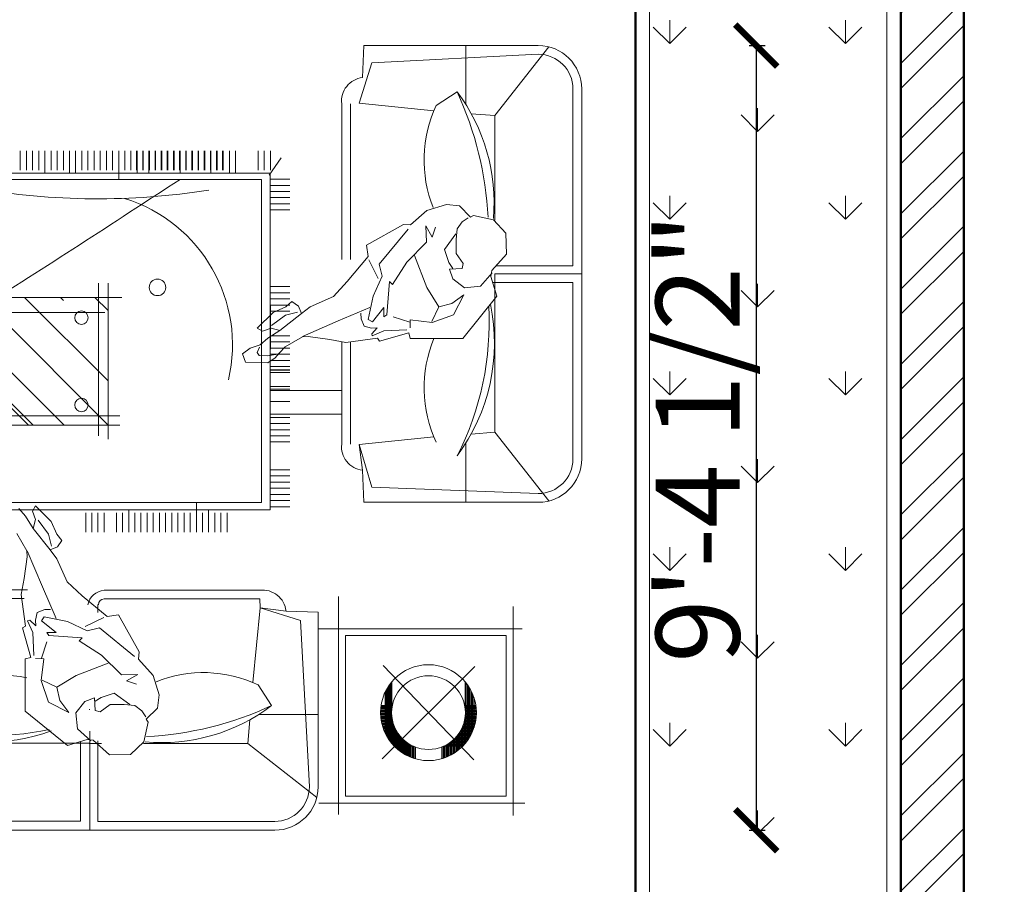
# Model space of a CAD drawing. Units: inches. Extents: x 261 to 2725, y 291 to 1454.
# Tile 31 of 35: x 2359 to 2500, y 546 to 670. Entities that reach past the tile are written whole.
import ezdxf

# ---------------------------------------------------------------- set-up
doc = ezdxf.new("R2010")
doc.units = ezdxf.units.IN
for name, color, linetype, lineweight in [('A-ANNO-DIMS', 136, 'Continuous', 18), ('A-FURN', 30, 'Continuous', 18), ('A-PLNT', 3, 'Continuous', 18), ('A-PLNT-PATT', 3, 'Continuous', 13), ('A-WALL', 222, 'Continuous', 50), ('A-WALL-PATT', 243, 'Continuous', 13)]:
    doc.layers.add(name, color=color, linetype=linetype, lineweight=lineweight)
doc.styles.get("Standard").update_dxf_attribs({"font": 'arial.ttf'})
doc.dimstyles.new('ISO-25', dxfattribs={"dimtxt": 12, "dimasz": 6, "dimexe": 1.25, "dimexo": 0.625, "dimtad": 1, "dimdec": 0, "dimlunit": 3, "dimtxsty": 'Standard', "dimblk": 'ARCHTICK', "dimcen": 2.5, "dimadec": 0, "dimazin": 0, "dimtfac": 1, "dimtdec": 0, "dimtmove": 0, "dimatfit": 3, "dimfxl": 1, "dimfxlon": 1, "dimarcsym": 0})

# ---------------------------------------------------------------- blocks, each defined once
blk = doc.blocks.new('A$C4DC51D13')
for p, q in [((3265.3, 2996.2), (1188.4, 2996.2)), ((2559.6, 2996.2), (2559.6, 2617.8)), ((1928.3, 2961.6), (2524.2, 2961.6)), ((2524.2, 2961.6), (2524.2, 2658.6)), ((2590.4, 2962.7), (2590.4, 2654.5)), ((3265.3, 2962.7), (2590.4, 2962.7)), ((3509.6, 2103.5), (3509.6, 2936.7)), ((4175.2, 2939.6), (4175.2, 2141.8)), ((3163.3, 2664.8), (3425.7, 2870.9)), ((3434.4, 2892.3), (4220.4, 2892.3)), ((3536.2, 2253.3), (3536.2, 2865.7)), ((3536.2, 2865.7), (4148.5, 2865.7)), ((4148.5, 2865.7), (4148.5, 2253.3)), ((3397.7, 2830.3), (3364.5, 2194.8)), ((3430.8, 2163.8), (3430.8, 2830.3)), ((4028.9, 2370.8), (3676, 2723.7)), ((4025.2, 2727.4), (3679.8, 2367.1)), ((3763, 2655.8), (3763, 2706.9)), ((3764.4, 2657), (3764.4, 2707.7)), ((3767.2, 2659.2), (3767.2, 2709.2)), ((3768.7, 2660.3), (3768.7, 2709.9)), ((3771.5, 2662.3), (3771.5, 2711.3)), ((3772.9, 2663.3), (3772.9, 2712)), ((3775.7, 2665.1), (3775.7, 2713.4)), ((3777.1, 2666.1), (3777.1, 2714)), ((3779.9, 2667.8), (3779.9, 2715.2)), ((3781.4, 2668.6), (3781.4, 2715.9)), ((3784.1, 2670.2), (3784.1, 2717)), ((3785.6, 2671), (3785.6, 2717.6)), ((3789.8, 2673.2), (3789.8, 2719.2)), ((3794, 2675.2), (3794, 2720.7)), ((3798.3, 2677.1), (3798.3, 2722)), ((3802.5, 2678.8), (3802.5, 2723.3)), ((3903.9, 2678.2), (3903.9, 2722.9)), ((3908.1, 2676.5), (3908.1, 2721.6)), ((3912.4, 2674.6), (3912.4, 2720.2)), ((3916.6, 2672.5), (3916.6, 2718.7)), ((3920.8, 2670.2), (3920.8, 2717)), ((3925.1, 2667.8), (3925.1, 2715.2)), ((3929.3, 2665.1), (3929.3, 2713.4)), ((3933.5, 2662.3), (3933.5, 2711.3)), ((3937.7, 2659.2), (3937.7, 2709.2)), ((3942, 2655.8), (3942, 2706.9)), ((3716.5, 2583.3), (3716.5, 2669.7)), ((3718, 2588.4), (3718, 2671.3)), ((3718.1, 2671.5), (3786.5, 2671.5)), ((3786.5, 2671.5), (3718.1, 2671.5)), ((3720.7, 2596.6), (3720.7, 2674.3)), ((3722.2, 2600.3), (3722.2, 2675.7)), ((3795.2, 2675.7), (3722.2, 2675.7)), ((3725, 2606.7), (3725, 2678.5)), ((3726.4, 2609.7), (3726.4, 2679.9)), ((3729.2, 2615), (3729.2, 2682.5)), ((3730.6, 2617.6), (3730.6, 2683.8)), ((3733.4, 2622.2), (3733.4, 2686.2)), ((3734.9, 2624.4), (3734.9, 2687.4)), ((3737.6, 2628.5), (3737.6, 2689.7)), ((3739.1, 2630.5), (3739.1, 2690.9)), ((3741.9, 2634.2), (3741.9, 2693)), ((3743.3, 2636), (3743.3, 2694.1)), ((3746.1, 2639.3), (3746.1, 2696.1)), ((3747.5, 2641), (3747.5, 2697.2)), ((3750.3, 2644), (3750.3, 2699.1)), ((3751.8, 2645.5), (3751.8, 2700)), ((3754.5, 2648.3), (3754.5, 2701.8)), ((3756, 2649.6), (3756, 2702.7)), ((3758.8, 2652.2), (3758.8, 2704.4)), ((3760.2, 2653.5), (3760.2, 2705.3)), ((3982.8, 2675.7), (3909.8, 2675.7)), ((3986.8, 2671.5), (3918.5, 2671.5)), ((3946.2, 2652.2), (3946.2, 2704.4)), ((3950.4, 2648.3), (3950.4, 2701.8)), ((3954.6, 2644), (3954.6, 2699.1)), ((3958.9, 2639.3), (3958.9, 2696.1)), ((3963.1, 2634.2), (3963.1, 2693)), ((3967.3, 2628.5), (3967.3, 2689.7)), ((3971.5, 2622.2), (3971.5, 2686.2)), ((3975.8, 2615), (3975.8, 2682.5)), ((3980, 2606.7), (3980, 2678.5)), ((3984.2, 2596.6), (3984.2, 2674.3)), ((3988.5, 2583.3), (3988.5, 2669.7)), ((1895.2, 2663.7), (2557.3, 2663.7)), ((2603.6, 2664.8), (2559, 2664.8)), ((3163.3, 2664.8), (2764.7, 2664.8)), ((3170.4, 2574.2), (3163.3, 2664.8)), ((3691.1, 2460.9), (3691.1, 2633.6)), ((3691.1, 2633.5), (3741.3, 2633.5)), ((3741.3, 2633.5), (3691.1, 2633.5)), ((3692.6, 2458.3), (3692.6, 2636.3)), ((3693.4, 2637.7), (3744.7, 2637.7)), ((3744.7, 2637.7), (3693.4, 2637.7)), ((3695.4, 2453.4), (3695.4, 2641.1)), ((3695.9, 2641.9), (3748.4, 2641.9)), ((3748.4, 2641.9), (3695.9, 2641.9)), ((3696.8, 2451.1), (3696.8, 2643.5)), ((3698.5, 2646.1), (3752.4, 2646.1)), ((3752.4, 2646.1), (3698.5, 2646.1)), ((3699.6, 2446.7), (3699.6, 2647.8)), ((3701, 2444.5), (3701, 2650)), ((3701.3, 2650.4), (3756.8, 2650.4)), ((3756.8, 2650.4), (3701.3, 2650.4)), ((3703.8, 2440.6), (3703.8, 2654)), ((3704.3, 2654.6), (3761.5, 2654.6)), ((3761.5, 2654.6), (3704.3, 2654.6)), ((3705.3, 2438.6), (3705.3, 2656)), ((3707.4, 2658.8), (3766.8, 2658.8)), ((3766.8, 2658.8), (3707.4, 2658.8)), ((3708.1, 2434.9), (3708.1, 2659.6)), ((3709.5, 2433.1), (3709.5, 2661.5)), ((3710.8, 2663.1), (3772.6, 2663.1)), ((3772.6, 2663.1), (3710.8, 2663.1)), ((3712.3, 2558.8), (3712.3, 2664.9)), ((3713.7, 2570.4), (3713.7, 2666.6)), ((3714.3, 2667.3), (3779.1, 2667.3)), ((3779.1, 2667.3), (3714.3, 2667.3)), ((3990.6, 2667.3), (3925.9, 2667.3)), ((3994.2, 2663.1), (3932.4, 2663.1)), ((3997.5, 2658.8), (3938.2, 2658.8)), ((4000.7, 2654.6), (3943.4, 2654.6)), ((4003.7, 2650.4), (3948.2, 2650.4)), ((4006.5, 2646.1), (3952.5, 2646.1)), ((4009.1, 2641.9), (3956.5, 2641.9)), ((4011.6, 2637.7), (3960.2, 2637.7)), ((3963.1, 2667.3), (3963.1, 2633.5)), ((4013.9, 2633.5), (3963.7, 2633.5)), ((3992.7, 2558.8), (3992.7, 2664.9)), ((3996.9, 2434.9), (3996.9, 2659.6)), ((4001.1, 2440.6), (4001.1, 2654)), ((4005.4, 2446.7), (4005.4, 2647.8)), ((4009.6, 2453.4), (4009.6, 2641.1)), ((4013.8, 2460.9), (4013.8, 2633.6)), ((3675.9, 2595.4), (3720.3, 2595.4)), ((3677.2, 2599.7), (3721.9, 2599.7)), ((3678.5, 2603.9), (3723.7, 2603.9)), ((3679.9, 2608.1), (3725.6, 2608.1)), ((3681.5, 2612.3), (3727.8, 2612.3)), ((3683.1, 2616.6), (3730.1, 2616.6)), ((3684.9, 2620.8), (3732.5, 2620.8)), ((3686.8, 2625), (3735.2, 2625)), ((3686.9, 2469.3), (3686.9, 2625.2)), ((3688.4, 2466.3), (3688.4, 2628.2)), ((3688.9, 2629.2), (3738.2, 2629.2)), ((3738.2, 2629.2), (3688.9, 2629.2)), ((4016.1, 2629.2), (3966.8, 2629.2)), ((4018.1, 2625), (3969.7, 2625)), ((4020, 2620.8), (3972.4, 2620.8)), ((4021.8, 2616.6), (3974.9, 2616.6)), ((4023.5, 2612.3), (3977.2, 2612.3)), ((4025.1, 2608.1), (3979.3, 2608.1)), ((4026.5, 2603.9), (3981.3, 2603.9)), ((4027.8, 2599.7), (3983, 2599.7)), ((4029, 2595.4), (3984.7, 2595.4)), ((4018, 2469.3), (4018, 2625.2)), ((4022.3, 2479), (4022.3, 2615.5)), ((4026.5, 2490.7), (4026.5, 2603.9)), ((3669.8, 2557.4), (3712.2, 2557.4)), ((3670.1, 2561.6), (3712.5, 2561.6)), ((3670.4, 2565.8), (3713, 2565.8)), ((3670.9, 2570.1), (3713.7, 2570.1)), ((3671.5, 2574.3), (3714.4, 2574.3)), ((3672.2, 2578.5), (3715.3, 2578.5)), ((3673, 2582.7), (3716.4, 2582.7)), ((3673.9, 2587), (3717.5, 2587)), ((3674.8, 2591.2), (3718.8, 2591.2)), ((4030.1, 2591.2), (3986.1, 2591.2)), ((4031.1, 2587), (3987.4, 2587)), ((4032, 2582.7), (3988.6, 2582.7)), ((4032.8, 2578.5), (3989.6, 2578.5)), ((4033.5, 2574.3), (3990.5, 2574.3)), ((4034, 2570.1), (3991.3, 2570.1)), ((4034.5, 2565.8), (3991.9, 2565.8)), ((4034.9, 2561.6), (3992.4, 2561.6)), ((4035.2, 2557.4), (3992.8, 2557.4)), ((2559, 2535.8), (2557.3, 2535.8)), ((3253.7, 2520.5), (3201.8, 2440.8)), ((3430.8, 2554.4), (3204.1, 2554.4)), ((3669.5, 2548.9), (3711.8, 2548.9)), ((3669.5, 2544.7), (3711.8, 2544.7)), ((3669.6, 2553.2), (3711.9, 2553.2)), ((3669.6, 2540.5), (3712, 2540.5)), ((3669.8, 2536.3), (3712.2, 2536.3)), ((3670.1, 2532), (3712.6, 2532)), ((3670.5, 2527.8), (3713.2, 2527.8)), ((3671, 2523.6), (3713.8, 2523.6)), ((3671.6, 2519.4), (3714.6, 2519.4)), ((3712.3, 2429.7), (3712.3, 2535.7)), ((4033.3, 2519.4), (3990.4, 2519.4)), ((4033.9, 2523.6), (3991.1, 2523.6)), ((4034.4, 2527.8), (3991.8, 2527.8)), ((4034.8, 2532), (3992.3, 2532)), ((4035.1, 2536.3), (3992.7, 2536.3)), ((3992.7, 2429.7), (3992.7, 2535.7)), ((4035.4, 2553.2), (3993, 2553.2)), ((4035.3, 2540.5), (3993, 2540.5)), ((4035.5, 2548.9), (3993.1, 2548.9)), ((4035.5, 2544.7), (3993.1, 2544.7)), ((3210.5, 2146.7), (3181.5, 2431.8)), ((4209.7, 2226.7), (3434.4, 2226.7)), ((4148.5, 2253.3), (3536.2, 2253.3)), ((3364.5, 2194.8), (3210.5, 2146.7)), ((2590.4, 2164.3), (2590.4, 2134)), ((3208.9, 2113), (3210.5, 2146.7)), ((3308.6, 2159.3), (3210.5, 2146.7)), ((3308.6, 2159.3), (3430.8, 2163.8)), ((2308.5, 2111.9), (1950.4, 2111.9)), ((2614.2, 2113), (3208.9, 2113)), ((2322.1, 2078.8), (1950.4, 2078.8)), ((2614.2, 2079.9), (3208.9, 2079.9)), ((2543.7, 1784.3), (2543.7, 1858.2)), ((2567.1, 1784.3), (2567.1, 1858.2)), ((2590.6, 1784.3), (2590.6, 1858.2)), ((2614.1, 1784.3), (2614.1, 1858.2)), ((2661, 1784.3), (2661, 1858.2)), ((2684.5, 1784.3), (2684.5, 1858.2)), ((2708, 1772.3), (2708, 1858.2)), ((2731.5, 1784.3), (2731.5, 1858.2)), ((2754.9, 1784.3), (2754.9, 1858.2)), ((2778.4, 1784.3), (2778.4, 1858.2)), ((2801.9, 1784.3), (2801.9, 1858.2)), ((2825.4, 1784.3), (2825.4, 1858.2)), ((2848.8, 1784.3), (2848.8, 1858.2)), ((2872.3, 1784.3), (2872.3, 1858.2)), ((2895.8, 1784.3), (2895.8, 1858.2)), ((2919.3, 1784.3), (2919.3, 1858.2)), ((2942.7, 1784.3), (2942.7, 1858.2)), ((2966.2, 1744.8), (2966.2, 1858.2)), ((2989.7, 1784.3), (2989.7, 1858.2)), ((3013.2, 1772.3), (3013.2, 1858.2)), ((3036.6, 1784.3), (3036.6, 1858.2)), ((3060.1, 1784.3), (3060.1, 1858.2)), ((3083.6, 1784.3), (3083.6, 1858.2)), ((3248.4, 1772.3), (1158.5, 1772.3)), ((3248.4, 487.7), (3248.4, 1772.3)), ((1196, 1744.8), (3215.6, 1744.8)), ((3215.6, 511), (3215.6, 1744.8)), ((3248.8, 1760.8), (3322.7, 1760.8)), ((3248.8, 1737.3), (3322.7, 1737.3)), ((3600.6, 1621.7), (3605.1, 1743.8)), ((3605.1, 1743.8), (4271.6, 1743.8)), ((3995.7, 1743.8), (3995.7, 1517.1)), ((4106.1, 1476.4), (4312.2, 1738.8)), ((3248.8, 1713.8), (3322.7, 1713.8)), ((4271.6, 1710.7), (3636.1, 1685.8)), ((3248.8, 1690.4), (3322.7, 1690.4)), ((3248.8, 1666.9), (3322.7, 1666.9)), ((3636.1, 1685.8), (3588, 1523.6)), ((3248.8, 1643.4), (3322.7, 1643.4)), ((3248.8, 1619.9), (3322.7, 1619.9)), ((3600.6, 1621.7), (3588, 1523.6)), ((4404, 1578.3), (4404, 904.6)), ((4437.5, 165.9), (4437.5, 1578.3)), ((3248.8, 1513.8), (3322.7, 1513.8)), ((3248.8, 1513.3), (3322.7, 1513.3)), ((3521.2, 1130.7), (3521.2, 1521.9)), ((3554.3, 1131.4), (3554.3, 1521.9)), ((3588, 1523.6), (3873.1, 1494.5)), ((2593.1, 907.9), (2593.1, 1490.3)), ((2629.1, 907.9), (2629.1, 1503.1)), ((3248.8, 1490.4), (3322.7, 1490.4)), ((3248.8, 1489.9), (3322.7, 1489.9)), ((3248.8, 1466.9), (3322.7, 1466.9)), ((4015.5, 1483.4), (4106.1, 1476.4)), ((4106.1, 1476.4), (4106.1, 872.1)), ((2674.6, 1449.9), (1641, 1449.9)), ((2343.3, 1449.9), (1855.3, 961.9)), ((2629.1, 1449), (2142, 961.9)), ((2325.1, 1449.9), (2154.2, 1279.1)), ((2461.6, 1449.9), (2177, 1165.3)), ((3248.8, 1443.4), (3322.7, 1443.4)), ((2674.6, 1413.9), (1641, 1413.9)), ((3248.8, 1419.9), (3322.7, 1419.9)), ((3250, 1407.8), (3519, 1407.8)), ((3248.8, 1359), (3322.7, 1359)), ((3248.8, 990.8), (3248.4, 1328.4)), ((3250, 1317.8), (3519, 1317.8)), ((2629.1, 1280.5), (2310.5, 961.9)), ((3248.8, 1312.1), (3322.7, 1312.1)), ((3248.8, 1302.3), (3322.7, 1302.3)), ((3248.8, 1249), (3322.7, 1249)), ((3248.8, 1248.5), (3322.7, 1248.5)), ((3248.8, 1239.3), (3322.7, 1239.3)), ((3248.8, 1238.8), (3322.7, 1238.8)), ((3248.8, 1225.5), (3322.7, 1225.5)), ((3248.8, 1202.1), (3322.7, 1202.1)), ((3248.8, 1178.6), (3322.7, 1178.6)), ((3248.8, 1155.1), (3322.7, 1155.1)), ((3248.8, 1131.6), (3322.7, 1131.6)), ((3248.8, 1108.2), (3322.7, 1108.2)), ((1648.3, 1019.6), (2616.7, 1019.6)), ((2629.1, 1012), (2579, 961.9)), ((3248.8, 1014.3), (3322.7, 1014.3)), ((3248.8, 990.8), (3322.7, 990.8)), ((1648.3, 961.9), (2681.9, 961.9)), ((2459.2, 974.1), (2447, 961.9)), ((3248.8, 967.3), (3322.7, 967.3)), ((3248.8, 943.8), (3322.7, 943.8)), ((3248.8, 920.4), (3322.7, 920.4)), ((4097.4, 904.6), (4404, 904.6)), ((4106.1, 871.5), (4437.5, 871.5)), ((4404, 840.7), (4110.5, 840.7)), ((4404, 165.9), (4404, 840.7)), ((3521.2, 816.9), (3521.2, 222.3)), ((3554.3, 816.9), (3554.3, 222.3)), ((4106.1, 267.8), (4106.1, 666.5)), ((3248.8, 627.8), (3322.7, 627.8)), ((3248.8, 604.4), (3322.7, 604.4)), ((3248.8, 580.9), (3322.7, 580.9)), ((3248.8, 557.4), (3322.7, 557.4)), ((3248.8, 533.9), (3322.7, 533.9)), ((3215.6, 511), (1196, 511)), ((2669.8, 511), (2669.8, 402.4)), ((3244.9, 495.1), (3290.3, 429)), ((3248.8, 510.5), (3322.7, 510.5)), ((1158.5, 487.7), (3248.4, 487.7)), ((2294.2, 476.3), (2294.2, 402.4)), ((2317.7, 476.3), (2317.7, 402.4)), ((2341.1, 476.3), (2341.1, 402.4)), ((2364.6, 476.3), (2364.6, 402.4)), ((2388.1, 487.7), (2388.1, 402.4)), ((2411.6, 476.3), (2411.6, 402.4)), ((2435, 476.3), (2435, 402.4)), ((2458.5, 476.3), (2458.5, 402.4)), ((2482, 487.7), (2482, 402.4)), ((2505.5, 487.7), (2505.5, 402.4)), ((2528.9, 476.3), (2528.9, 402.4)), ((2552.4, 476.3), (2552.4, 402.4)), ((2575.9, 476.3), (2575.9, 402.4)), ((2599.4, 476.3), (2599.4, 402.4)), ((2622.8, 476.3), (2622.8, 402.4)), ((2646.3, 476.3), (2646.3, 402.4)), ((2693.3, 476.3), (2693.3, 402.4)), ((2716.7, 476.3), (2716.7, 402.4)), ((2738, 476.3), (2738, 402.4)), ((2740.2, 487.7), (2740.2, 402.4)), ((2761.5, 476.3), (2761.5, 402.4)), ((2763.7, 476.3), (2763.7, 402.4)), ((2784.9, 487.7), (2784.9, 402.4)), ((2787.2, 476.3), (2787.2, 402.4)), ((2808.4, 476.3), (2808.4, 402.4)), ((2810.6, 476.3), (2810.6, 402.4)), ((2831.9, 476.3), (2831.9, 402.4)), ((2834.1, 476.3), (2834.1, 402.4)), ((2855.4, 476.3), (2855.4, 402.4)), ((2857.6, 476.3), (2857.6, 402.4)), ((2878.8, 476.3), (2878.8, 402.4)), ((2881.1, 476.3), (2881.1, 402.4)), ((2902.3, 476.3), (2902.3, 402.4)), ((2904.5, 487.7), (2904.5, 402.4)), ((2925.8, 476.3), (2925.8, 402.4)), ((2928, 476.3), (2928, 402.4)), ((2949.3, 476.3), (2949.3, 402.4)), ((2951.5, 476.3), (2951.5, 402.4)), ((2972.7, 476.3), (2972.7, 402.4)), ((2975, 476.3), (2975, 402.4)), ((2996.2, 476.3), (2996.2, 402.4)), ((2998.4, 476.3), (2998.4, 402.4)), ((3019.7, 476.3), (3019.7, 402.4)), ((3021.9, 487.7), (3021.9, 402.4)), ((3043.2, 476.3), (3043.2, 402.4)), ((3045.4, 476.3), (3045.4, 402.4)), ((3066.6, 476.3), (3066.6, 402.4)), ((3068.9, 476.3), (3068.9, 402.4)), ((3092.3, 476.3), (3092.3, 402.4)), ((3092.7, 484.5), (3092.7, 410.6)), ((3115.8, 476.3), (3115.8, 402.4)), ((3116.2, 484.5), (3116.2, 410.6)), ((3202.2, 476.3), (3202.2, 402.4)), ((3225.7, 476.3), (3225.7, 402.4)), ((3249.2, 476.3), (3249.2, 402.4)), ((4015.5, 260.8), (4106.1, 267.8)), ((4106.1, 267.8), (4312.2, 5.4)), ((3588, 220.6), (3873.1, 249.7)), ((3961.8, 177.4), (3882.1, 229.3)), ((3995.7, 0.4), (3995.7, 227)), ((3636.1, 66.6), (3588, 220.6)), ((3600.6, 122.5), (3605.1, 0.4)), ((4271.6, 33.5), (3636.1, 66.6)), ((3605.1, 0.4), (4271.6, 0.4))]:
    blk.add_line(p, q)
at = {"linetype": 'ByBlock'}
for points in [[(2288.6, 1768), (2313.7, 1797.6), (2342.9, 1843.9), (2352.5, 1810.4), (2340.1, 1777.7), (2351.8, 1757), (2412.3, 1818), (2433.1, 1866.4), (2453.1, 1889.5), (2436, 1914.7), (2407.6, 1926.2), (2433.7, 1959.9), (2473.1, 2048.3), (2530.6, 2101.1), (2625.9, 2180.3), (2669, 2174.2), (2748.1, 2315.4), (2745.8, 2342.6), (2801.2, 2404.9), (2823.9, 2479.6), (2818.4, 2529.9), (2775.1, 2571.7), (2782.4, 2583.3), (2765.2, 2658.8), (2714.5, 2706.9), (2634.6, 2708.6), (2571.9, 2652.6), (2548.8, 2649.4), (2474, 2672.1), (2312.9, 2542.1), (2312.9, 2341.6), (2333.9, 2336.4), (2302, 2223.9), (2313.6, 2216.6), (2297.4, 2095.7), (2309.3, 2034.9), (2320.2, 1952), (2319.3, 1929.9), (2280.8, 1863.6)], [(2563.4, 2654.7), (2512.2, 2609.3), (2506.2, 2548.3), (2540.1, 2504.4), (2576.9, 2490.9), (2579.8, 2539.3), (2598.7, 2543.6), (2636.7, 2516.4), (2690.3, 2516.7), (2731.2, 2520.1), (2758.5, 2540.1), (2773, 2563.3)], [(2629.1, 2357.8), (2507, 2405.5), (2433.2, 2450.3), (2445.5, 2500.8), (2478.9, 2546.1), (2402.4, 2506.9), (2373.4, 2424.8), (2384.4, 2341.9), (2352.8, 2340.7)], [(2712.3, 2515.8), (2652.7, 2472.4), (2603.2, 2489), (2580, 2503.6)], [(2433.2, 2450.3), (2377.6, 2423.8)], [(2738, 2438.2), (2699.2, 2425.4), (2742.4, 2401.4), (2680.4, 2403.2), (2604.1, 2328.3), (2519.2, 2273.3), (2529.8, 2261.8), (2402.7, 2252.7), (2395.4, 2241.1), (2431.1, 2241.3), (2375.7, 2196.9), (2385.2, 2181.2), (2474.4, 2199.5), (2549.9, 2234.6), (2596.2, 2223.2), (2730.1, 2333.1)], [(2374.9, 2339.8), (2395.2, 2276.9)], [(2409.5, 2153), (2387.5, 2153.9), (2359, 2165.4), (2352.6, 2193.7), (2353.5, 2215.7), (2330.5, 2194.6), (2322.1, 2196.7), (2341.8, 2240.9), (2345.5, 2329.1)], [(2613.2, 2183.4), (2541.6, 2218.8)], [(2431.4, 2187.8), (2379.5, 2066.7), (2320.2, 1929.7)], [(2407.6, 1926.2), (2342.9, 1843.9)], [(2412.9, 1911.5), (2401.6, 1865.2), (2361.9, 1812.5)], [(3207.2, 1152), (3198.7, 1171.9), (3206, 1183.5), (3237.5, 1184.7), (3284.8, 1177.6)], [(3629.1, 999.7), (3508, 1051.6), (3371, 1110.9)], [(3594.3, 1021.6), (3595.2, 1043.7), (3606.7, 1072.1), (3635, 1078.6), (3657, 1077.6), (3635.9, 1100.6), (3638, 1109.1), (3682.2, 1089.3), (3770.4, 1085.6)], [(3352.8, 1018.2), (3306.5, 1029.5), (3253.8, 1069.2)], [(3367.5, 1023.6), (3285.2, 1088.3)], [(3879.5, 693.2), (3866.7, 732), (3842.7, 688.8), (3844.5, 750.8), (3769.6, 827.1), (3714.6, 911.9), (3703.1, 901.3), (3694, 1028.4), (3682.4, 1035.7), (3682.6, 1000), (3638.2, 1055.5), (3622.5, 1045.9), (3640.8, 956.7), (3675.9, 881.2), (3664.5, 834.9), (3774.4, 701)], [(3781.1, 1056.2), (3718.2, 1035.9)], [(3799.1, 802), (3846.8, 924.2), (3891.6, 998), (3942.1, 985.6), (3987.4, 952.2), (3948.2, 1028.7), (3866.1, 1057.7), (3783.2, 1046.8), (3782, 1078.3)], [(3891.6, 998), (3865.1, 1053.5)], [(4096, 867.7), (4050.6, 918.9), (3989.6, 924.9), (3945.7, 891.1), (3932.2, 854.2), (3980.6, 851.3), (3984.9, 832.4), (3957.7, 794.4), (3958, 740.9), (3961.4, 699.9), (3981.4, 672.7), (4004.6, 658.1)], [(3624.7, 817.9), (3660.1, 889.6)], [(3957.1, 718.8), (3913.7, 778.5), (3930.3, 827.9), (3944.9, 851.1)]]:
    blk.add_lwpolyline(points, dxfattribs=at)
blk.add_lwpolyline([(3285.2, 1088.3), (3251.7, 1078.6), (3219, 1091.1), (3198.3, 1079.4), (3259.3, 1018.8), (3307.7, 998), (3330.8, 978), (3356, 995.1), (3367.5, 1023.6), (3401.2, 997.5), (3489.6, 958), (3542.4, 900.5), (3621.6, 805.3), (3615.5, 762.2), (3756.7, 683), (3783.9, 685.3), (3846.2, 629.9), (3920.9, 607.2), (3971.2, 612.7), (4013, 656), (4024.6, 648.7), (4100.1, 665.9), (4148.2, 716.6), (4149.9, 796.5), (4093.9, 859.3), (4090.7, 882.4), (4113.4, 957.1), (3983.4, 1118.2), (3782.9, 1118.2), (3777.7, 1097.2), (3665.2, 1129.2), (3657.9, 1117.6), (3537, 1133.7), (3476.2, 1121.9), (3393.3, 1110.9), (3371.2, 1111.9), (3304.9, 1150.4), (3283.7, 1173.4), (3267, 1191.9), (3239.5, 1211), (3154.4, 1209.5), (3142, 1176.8), (3171.1, 1155.3), (3209.3, 1142.5), (3238.9, 1117.5)], close=True, dxfattribs=at)
for centre, radius in [((3852.5, 2547.3), 183), ((3852.5, 2547.3), 140.7), ((2527.6, 1372.6), 25.7), ((2527.6, 1039.3), 25.7), ((2817.9, 923.4), 31.7)]:
    blk.add_circle(centre, radius)
for centre, radius, start, end in [((3265.3, 2830.3), 165.9, 0, 90), ((3265.3, 2830.3), 132.4, 0, 90), ((2210.2, 1780.8), 852.5, 76.866, 111.6839), ((2192.2, 2032.6), 624.6, 69.4145, 118.3621), ((2633.9, 373.6), 2292.5, 91.8726, 91.9144), ((2832.8, 1963.1), 698.5, 52.9389, 95.0789), ((2713.3, 1357.7), 1282.3, 65.0725, 87.2152), ((2216, 2892.1), 488.4, 234.4888, 282.1285), ((2993.8, 2882.7), 488.4, 248.2152, 295.2134), ((3219.2, 2169.3), 90, 263.4179, 353.5749), ((2619.6, 2148.3), 68.5, 191.0595, 265.4426), ((2614.2, 2135.1), 22.1, 180, 270), ((4271.6, 1578.3), 165.9, 0, 90), ((4271.6, 1578.3), 132.4, 0, 90), ((3610.6, 1532.2), 90, 96.4251, 186.5821), ((3383, 1136.2), 721.4, 348.1046, 36.6442), ((2968.3, 1058.8), 1115.8, 356.7543, 27.0804), ((4324, 1306.8), 488.4, 154.7866, 202.7137), ((2517.5, 1143.6), 586.7, 287.3395, 13.1463), ((-29968.2, -49615.7), 59944, 56.743614, 57.623407), ((3404.4, 598.4), 698.5, 322.9389, 5.0789), ((2799, 717.9), 1282.3, 335.0725, 357.2152), ((4324, 437.4), 488.4, 158.2152, 205.2134), ((2591.9, -2109.1), 2694.5, 80.9842, 100.0261), ((3610.6, 212), 90, 173.4179, 263.5749), ((4271.6, 165.9), 132.4, 270, 0), ((4271.6, 165.9), 165.9, 270, 0)]:
    blk.add_arc(centre, radius, start, end)
blk = doc.blocks.new('_ArchTick')
at = {"color": 0, "linetype": 'ByBlock', "const_width": 0.15}
blk.add_lwpolyline([(-0.5, -0.5), (0.5, 0.5)], dxfattribs=at)
blk = doc.blocks.new('*D71')
at = {"layer": 'A-ANNO-DIMS', "color": 0, "lineweight": -2, "ltscale": 0.07, "transparency": 16777216}
for p, q in [((2272.38, 690.06), (2272.38, 692.31)), ((2439.01, 690.06), (2439.01, 692.31)), ((2272.38, 691.06), (2439.01, 691.06)), ((2439.01, 691.06), (2725.34, 691.06))]:
    blk.add_line(p, q, dxfattribs=at)
at = {"layer": 'Defpoints', "color": 0, "ltscale": 0.07, "transparency": 16777216}
for p in [(2439.01, 691.06), (2272.38, 666.07), (2439.01, 666.07)]:
    blk.add_point(p, dxfattribs=at)
at = {"layer": 'A-ANNO-DIMS', "color": 0, "lineweight": -2, "ltscale": 0.07, "transparency": 16777216, "xscale": 6, "yscale": 6, "zscale": 6, "rotation": 180}
blk.add_blockref('_ArchTick', (2272.38, 691.06), dxfattribs=at)
at = {"layer": 'A-ANNO-DIMS', "color": 0, "lineweight": -2, "ltscale": 0.07, "transparency": 16777216, "xscale": 6, "yscale": 6, "zscale": 6}
blk.add_blockref('_ArchTick', (2439.01, 691.06), dxfattribs=at)
at = {"layer": 'A-ANNO-DIMS', "color": 0, "ltscale": 0.07, "transparency": 16777216, "insert": (2585.18, 697.9), "char_height": 12, "attachment_point": 5}
blk.add_mtext('TERRACE SEATING SET 13\'-10 1/2"', dxfattribs=at)
blk = doc.blocks.new('*D72')
at = {"layer": 'A-ANNO-DIMS', "color": 0, "lineweight": -2, "ltscale": 0.07, "transparency": 16777216}
for p, q in [((2463.01, 666.07), (2465.26, 666.07)), ((2464.01, 666.07), (2464.01, 553.71)), ((2463.01, 553.71), (2465.26, 553.71))]:
    blk.add_line(p, q, dxfattribs=at)
at = {"layer": 'Defpoints', "color": 0, "ltscale": 0.07, "transparency": 16777216}
for p in [(2439.01, 666.07), (2439.01, 553.71), (2464.01, 553.71)]:
    blk.add_point(p, dxfattribs=at)
at = {"layer": 'A-ANNO-DIMS', "color": 0, "lineweight": -2, "ltscale": 0.07, "transparency": 16777216, "xscale": 6, "yscale": 6, "zscale": 6}
for p, rotation in [((2464.01, 666.07), 90), ((2464.01, 553.71), 270)]:
    blk.add_blockref('_ArchTick', p, dxfattribs=dict(at, rotation=rotation))
at = {"layer": 'A-ANNO-DIMS', "color": 0, "ltscale": 0.07, "transparency": 16777216, "insert": (2457.18, 609.89), "char_height": 12, "attachment_point": 5, "rotation": 90}
blk.add_mtext('9\'-4 1/2"', dxfattribs=at)
blk = doc.blocks.new('*D82')
at = {"layer": 'A-ANNO-DIMS', "color": 0, "lineweight": -2, "ltscale": 0.07, "transparency": 16777216}
for p, q in [((2600.96, 679.47), (2603.21, 679.47)), ((2601.96, 517.47), (2601.96, 679.47)), ((2600.96, 517.47), (2603.21, 517.47))]:
    blk.add_line(p, q, dxfattribs=at)
at = {"layer": 'Defpoints', "color": 0, "ltscale": 0.07, "transparency": 16777216}
for p in [(946.45, 679.47), (2601.96, 679.47), (946.45, 517.47)]:
    blk.add_point(p, dxfattribs=at)
at = {"layer": 'A-ANNO-DIMS', "color": 0, "lineweight": -2, "ltscale": 0.07, "transparency": 16777216, "xscale": 6, "yscale": 6, "zscale": 6}
for p, rotation in [((2601.96, 679.47), 90), ((2601.96, 517.47), 270)]:
    blk.add_blockref('_ArchTick', p, dxfattribs=dict(at, rotation=rotation))
at = {"layer": 'A-ANNO-DIMS', "color": 0, "ltscale": 0.07, "transparency": 16777216, "insert": (2595.2, 598.47), "char_height": 12, "attachment_point": 5, "rotation": 90}
blk.add_mtext('13\'-6"', dxfattribs=at)
blk = doc.blocks.new('*D111')
at = {"layer": 'A-ANNO-DIMS', "color": 0, "lineweight": -2, "ltscale": 0.07, "transparency": 16777216}
for p, q in [((2600.96, 550.47), (2603.21, 550.47)), ((2601.96, 448.47), (2601.96, 550.47)), ((2600.96, 448.47), (2603.21, 448.47))]:
    blk.add_line(p, q, dxfattribs=at)
at = {"layer": 'Defpoints', "color": 0, "ltscale": 0.07, "transparency": 16777216}
for p in [(1720.08, 550.47), (2601.96, 550.47), (1720.08, 448.47)]:
    blk.add_point(p, dxfattribs=at)
at = {"layer": 'A-ANNO-DIMS', "color": 0, "lineweight": -2, "ltscale": 0.07, "transparency": 16777216, "xscale": 6, "yscale": 6, "zscale": 6}
for p, rotation in [((2601.96, 550.47), 90), ((2601.96, 448.47), 270)]:
    blk.add_blockref('_ArchTick', p, dxfattribs=dict(at, rotation=rotation))
at = {"layer": 'A-ANNO-DIMS', "color": 0, "ltscale": 0.07, "transparency": 16777216, "insert": (2595.21, 499.47), "char_height": 12, "attachment_point": 5, "rotation": 90}
blk.add_mtext('8\'-6"', dxfattribs=at)
blk = doc.blocks.new('*D112')
at = {"layer": 'A-ANNO-DIMS', "color": 0, "lineweight": -2, "ltscale": 0.07, "transparency": 16777216}
for p, q in [((2600.96, 679.47), (2603.21, 679.47)), ((2601.96, 550.47), (2601.96, 679.47)), ((2600.96, 550.47), (2603.21, 550.47))]:
    blk.add_line(p, q, dxfattribs=at)
at = {"layer": 'Defpoints', "color": 0, "ltscale": 0.07, "transparency": 16777216}
for p in [(1720.08, 679.47), (2601.96, 679.47), (1720.08, 550.47)]:
    blk.add_point(p, dxfattribs=at)
at = {"layer": 'A-ANNO-DIMS', "color": 0, "lineweight": -2, "ltscale": 0.07, "transparency": 16777216, "xscale": 6, "yscale": 6, "zscale": 6}
for p, rotation in [((2601.96, 679.47), 90), ((2601.96, 550.47), 270)]:
    blk.add_blockref('_ArchTick', p, dxfattribs=dict(at, rotation=rotation))
at = {"layer": 'A-ANNO-DIMS', "color": 0, "ltscale": 0.07, "transparency": 16777216, "insert": (2595.21, 614.97), "char_height": 12, "attachment_point": 5, "rotation": 90}
blk.add_mtext('10\'-9"', dxfattribs=at)
blk = doc.blocks.new('*D126')
at = {"layer": 'A-ANNO-DIMS', "color": 0, "lineweight": -2, "ltscale": 0.07, "transparency": 16777216}
for p, q in [((2600.96, 673.47), (2603.21, 673.47)), ((2601.96, 496.47), (2601.96, 673.47)), ((2600.96, 496.47), (2603.21, 496.47))]:
    blk.add_line(p, q, dxfattribs=at)
at = {"layer": 'Defpoints', "color": 0, "ltscale": 0.07, "transparency": 16777216}
for p in [(2484.71, 673.47), (2601.96, 673.47), (2493.71, 496.47)]:
    blk.add_point(p, dxfattribs=at)
at = {"layer": 'A-ANNO-DIMS', "color": 0, "lineweight": -2, "ltscale": 0.07, "transparency": 16777216, "xscale": 6, "yscale": 6, "zscale": 6}
for p, rotation in [((2601.96, 673.47), 90), ((2601.96, 496.47), 270)]:
    blk.add_blockref('_ArchTick', p, dxfattribs=dict(at, rotation=rotation))
at = {"layer": 'A-ANNO-DIMS', "color": 0, "ltscale": 0.07, "transparency": 16777216, "insert": (2595.21, 584.97), "char_height": 12, "attachment_point": 5, "rotation": 90}
blk.add_mtext('14\'-9"', dxfattribs=at)
blk = doc.blocks.new('*D131')
at = {"layer": 'A-ANNO-DIMS', "color": 0, "lineweight": -2, "ltscale": 0.07, "transparency": 16777216}
for p, q in [((2448.71, 305.22), (2448.71, 302.97)), ((2484.71, 305.22), (2484.71, 302.97)), ((2448.71, 304.22), (2484.71, 304.22))]:
    blk.add_line(p, q, dxfattribs=at)
at = {"layer": 'Defpoints', "color": 0, "ltscale": 0.07, "transparency": 16777216}
for p in [(2484.71, 673.47), (2448.71, 671.47), (2484.71, 304.22)]:
    blk.add_point(p, dxfattribs=at)
at = {"layer": 'A-ANNO-DIMS', "color": 0, "lineweight": -2, "ltscale": 0.07, "transparency": 16777216, "xscale": 6, "yscale": 6, "zscale": 6, "rotation": 180}
blk.add_blockref('_ArchTick', (2448.71, 304.22), dxfattribs=at)
at = {"layer": 'A-ANNO-DIMS', "color": 0, "lineweight": -2, "ltscale": 0.07, "transparency": 16777216, "xscale": 6, "yscale": 6, "zscale": 6}
blk.add_blockref('_ArchTick', (2484.71, 304.22), dxfattribs=at)
at = {"layer": 'A-ANNO-DIMS', "color": 0, "ltscale": 0.07, "transparency": 16777216, "insert": (2466.71, 310.97), "char_height": 12, "attachment_point": 5}
blk.add_mtext('3\'-0"', dxfattribs=at)
blk = doc.blocks.new('*D132')
at = {"layer": 'A-ANNO-DIMS', "color": 0, "lineweight": -2, "ltscale": 0.07, "transparency": 16777216}
for p, q in [((2364.21, 305.22), (2364.21, 302.97)), ((2484.71, 305.22), (2484.71, 302.97)), ((2364.21, 304.22), (2484.71, 304.22))]:
    blk.add_line(p, q, dxfattribs=at)
at = {"layer": 'Defpoints', "color": 0, "ltscale": 0.07, "transparency": 16777216}
for p in [(2364.21, 799.47), (2484.71, 799.47), (2484.71, 304.22)]:
    blk.add_point(p, dxfattribs=at)
at = {"layer": 'A-ANNO-DIMS', "color": 0, "lineweight": -2, "ltscale": 0.07, "transparency": 16777216, "xscale": 6, "yscale": 6, "zscale": 6, "rotation": 180}
blk.add_blockref('_ArchTick', (2364.21, 304.22), dxfattribs=at)
at = {"layer": 'A-ANNO-DIMS', "color": 0, "lineweight": -2, "ltscale": 0.07, "transparency": 16777216, "xscale": 6, "yscale": 6, "zscale": 6}
blk.add_blockref('_ArchTick', (2484.71, 304.22), dxfattribs=at)
at = {"layer": 'A-ANNO-DIMS', "color": 0, "ltscale": 0.07, "transparency": 16777216, "insert": (2424.46, 311.05), "char_height": 12, "attachment_point": 5}
blk.add_mtext('10\'-0 1/2"', dxfattribs=at)
blk = doc.blocks.new('*D136')
at = {"layer": 'A-ANNO-DIMS', "color": 0, "lineweight": -2, "ltscale": 0.07, "transparency": 16777216}
for p, q in [((2600.96, 675.78), (2603.21, 675.78)), ((2601.96, 675.78), (2601.96, 475.47)), ((2600.96, 475.47), (2603.21, 475.47))]:
    blk.add_line(p, q, dxfattribs=at)
at = {"layer": 'Defpoints', "color": 0, "ltscale": 0.07, "transparency": 16777216}
for p in [(2208.67, 675.78), (2208.67, 475.47), (2601.96, 475.47)]:
    blk.add_point(p, dxfattribs=at)
at = {"layer": 'A-ANNO-DIMS', "color": 0, "lineweight": -2, "ltscale": 0.07, "transparency": 16777216, "xscale": 6, "yscale": 6, "zscale": 6}
for p, rotation in [((2601.96, 675.78), 90), ((2601.96, 475.47), 270)]:
    blk.add_blockref('_ArchTick', p, dxfattribs=dict(at, rotation=rotation))
at = {"layer": 'A-ANNO-DIMS', "color": 0, "ltscale": 0.07, "transparency": 16777216, "insert": (2595.13, 575.62), "char_height": 12, "attachment_point": 5, "rotation": 90}
blk.add_mtext('16\'-8 1/2"', dxfattribs=at)
blk = doc.blocks.new('*D137')
at = {"layer": 'A-ANNO-DIMS', "color": 0, "lineweight": -2, "ltscale": 0.07, "transparency": 16777216}
for p, q in [((2600.96, 642.39), (2603.21, 642.39)), ((2601.96, 642.39), (2601.96, 634.05)), ((2600.96, 634.05), (2603.21, 634.05)), ((2601.96, 634.05), (2601.96, 566.94))]:
    blk.add_line(p, q, dxfattribs=at)
at = {"layer": 'Defpoints', "color": 0, "ltscale": 0.07, "transparency": 16777216}
for p in [(2221.19, 642.39), (2221.19, 634.05), (2601.96, 634.05)]:
    blk.add_point(p, dxfattribs=at)
at = {"layer": 'A-ANNO-DIMS', "color": 0, "lineweight": -2, "ltscale": 0.07, "transparency": 16777216, "xscale": 6, "yscale": 6, "zscale": 6}
for p, rotation in [((2601.96, 642.39), 90), ((2601.96, 634.05), 270)]:
    blk.add_blockref('_ArchTick', p, dxfattribs=dict(at, rotation=rotation))
at = {"layer": 'A-ANNO-DIMS', "color": 0, "ltscale": 0.07, "transparency": 16777216, "insert": (2595.13, 597.49), "char_height": 12, "attachment_point": 5, "rotation": 90}
blk.add_mtext('0\'-8 1/2"', dxfattribs=at)
blk = doc.blocks.new('*D138')
at = {"layer": 'A-ANNO-DIMS', "color": 0, "lineweight": -2, "ltscale": 0.07, "transparency": 16777216}
for p, q in [((2600.96, 634.05), (2603.21, 634.05)), ((2601.96, 634.05), (2601.96, 517.2)), ((2600.96, 517.2), (2603.21, 517.2))]:
    blk.add_line(p, q, dxfattribs=at)
at = {"layer": 'Defpoints', "color": 0, "ltscale": 0.07, "transparency": 16777216}
for p in [(2221.19, 634.05), (2221.19, 517.2), (2601.96, 517.2)]:
    blk.add_point(p, dxfattribs=at)
at = {"layer": 'A-ANNO-DIMS', "color": 0, "lineweight": -2, "ltscale": 0.07, "transparency": 16777216, "xscale": 6, "yscale": 6, "zscale": 6}
for p, rotation in [((2601.96, 634.05), 90), ((2601.96, 517.2), 270)]:
    blk.add_blockref('_ArchTick', p, dxfattribs=dict(at, rotation=rotation))
at = {"layer": 'A-ANNO-DIMS', "color": 0, "ltscale": 0.07, "transparency": 16777216, "insert": (2595.21, 575.62), "char_height": 12, "attachment_point": 5, "rotation": 90}
blk.add_mtext('9\'-9"', dxfattribs=at)

msp = doc.modelspace()

# ---------------------------------------------------------------- hatches: boundary and pattern name
at = {"layer": 'A-PLNT-PATT'}
h = msp.add_hatch(dxfattribs=at)
h.set_pattern_fill('GRASS', color=256, scale=0.7)
h.paths.add_polyline_path([(2052.71, 797.47), (2018.71, 797.47), (2018.71, 450.47), (2206.67, 450.47), (2206.67, 507.47), (2482.71, 507.47), (2482.71, 671.47), (2448.71, 671.47), (2448.71, 541.47), (2172.67, 541.47), (2172.67, 484.47), (2052.71, 484.47)])
at = {"layer": 'A-WALL-PATT'}
h = msp.add_hatch(dxfattribs=at)
h.set_pattern_fill('ANSI32', color=256, scale=0.8)
h.paths.add_polyline_path([(478.45, 685.47), (580.45, 685.47), (580.45, 691.47), (577.45, 691.47), (577.45, 694.47), (571.45, 694.47), (571.45, 691.47), (478.45, 691.47), (478.45, 721.47), (469.45, 721.47), (469.45, 508.47), (538.45, 508.47), (538.45, 517.47), (478.45, 517.47)])
h.paths.add_polyline_path([(694.45, 517.47), (676.45, 517.47), (676.45, 646.47), (670.45, 646.47), (670.45, 517.47), (610.45, 517.47), (610.45, 508.47), (694.45, 508.47)])
h.paths.add_polyline_path([(676.45, 784.47), (478.45, 784.47), (478.45, 844.47), (469.45, 844.47), (469.45, 745.47), (478.45, 745.47), (478.45, 775.47), (571.45, 775.47), (571.45, 724.47), (577.45, 724.47), (577.45, 775.47), (670.45, 775.47), (670.45, 691.47), (610.45, 691.47), (610.45, 685.47), (670.45, 685.47), (670.45, 682.47), (676.45, 682.47)])
h.paths.add_polyline_path([(955.45, 880.47), (946.45, 880.47), (946.45, 808.47), (778.45, 808.47), (778.45, 799.47), (946.45, 799.47), (946.45, 517.47), (898.45, 517.47), (898.45, 508.47), (955.45, 508.47)])
h.paths.add_polyline_path([(778.45, 598.47), (772.45, 598.47), (772.45, 517.47), (754.45, 517.47), (754.45, 508.47), (826.45, 508.47), (826.45, 517.47), (778.45, 517.47)])
h.paths.add_polyline_path([(955.45, 1090.47), (946.45, 1090.47), (946.45, 1030.47), (817.45, 1030.47), (817.45, 1024.47), (946.45, 1024.47), (946.45, 952.47), (955.45, 952.47)])
h.paths.add_polyline_path([(955.45, 1231.47), (730.45, 1231.47), (730.45, 1222.47), (772.45, 1222.47), (772.45, 1096.47), (766.45, 1096.47), (766.45, 1090.47), (772.45, 1090.47), (772.45, 1006.47), (712.45, 1006.47), (712.45, 1000.47), (778.45, 1000.47), (778.45, 1024.47), (781.45, 1024.47), (781.45, 1030.47), (778.45, 1030.47), (778.45, 1222.47), (946.45, 1222.47), (946.45, 1162.47), (955.45, 1162.47)])
h.paths.add_polyline_path([(694.45, 1231.47), (619.45, 1231.47), (619.45, 1222.47), (646.45, 1222.47), (646.45, 1039.47), (652.45, 1039.47), (652.45, 1090.47), (736.45, 1090.47), (736.45, 1096.47), (652.45, 1096.47), (652.45, 1222.47), (694.45, 1222.47)])
h.paths.add_polyline_path([(571.45, 1231.47), (469.45, 1231.47), (469.45, 1099.47), (478.45, 1099.47), (478.45, 1144.47), (544.45, 1144.47), (544.45, 1153.47), (538.45, 1153.47), (538.45, 1150.47), (478.45, 1150.47), (478.45, 1222.47), (538.45, 1222.47), (538.45, 1183.47), (544.45, 1183.47), (544.45, 1222.47), (571.45, 1222.47)])
h.paths.add_polyline_path([(538.45, 1006.47), (478.45, 1006.47), (478.45, 1051.47), (469.45, 1051.47), (469.45, 940.47), (478.45, 940.47), (478.45, 1000.47), (538.45, 1000.47)])
h.paths.add_polyline_path([(652.45, 1006.47), (652.45, 1009.47), (646.45, 1009.47), (646.45, 1006.47), (586.45, 1006.47), (586.45, 1000.47), (652.45, 1000.47)])
h.paths.add_polyline_path([(1288.08, 973.47), (1243.08, 973.47), (1243.08, 920.97), (1252.08, 920.97), (1252.08, 964.47), (1288.08, 964.47)], flags=17)
h.paths.add_polyline_path([(1402.08, 805.47), (1252.08, 805.47), (1252.08, 848.97), (1243.08, 848.97), (1243.08, 757.47), (1252.08, 757.47), (1252.08, 799.47), (1294.08, 799.47), (1372.08, 799.47), (1372.08, 779.47), (1372.08, 715.47), (1378.08, 715.47), (1378.08, 799.47), (1402.08, 799.47)])
h.paths.add_polyline_path([(1252.08, 721.47), (1243.08, 721.47), (1243.08, 439.47), (1729.08, 439.47), (1729.08, 709.47), (1720.08, 709.47), (1720.08, 679.47), (1582.08, 679.47), (1582.08, 670.47), (1588.08, 670.47), (1588.08, 673.47), (1720.08, 673.47), (1720.08, 559.47), (1690.08, 559.47), (1690.08, 550.47), (1720.08, 550.47), (1720.08, 448.47), (1252.08, 448.47), (1252.08, 496.47), (1312.08, 496.47), (1312.08, 505.47), (1252.08, 505.47), (1252.08, 673.47), (1405.08, 673.47), (1405.08, 679.47), (1378.08, 679.47), (1378.08, 685.47), (1372.08, 685.47), (1372.08, 679.47), (1252.08, 679.47)])
h.paths.add_polyline_path([(1450.08, 550.47), (1480.08, 550.47), (1480.08, 559.47), (1450.08, 559.47), (1450.08, 679.47), (1441.08, 679.47), (1441.08, 673.47), (1444.08, 673.47), (1444.08, 505.47), (1384.08, 505.47), (1384.08, 496.47), (1450.08, 496.47)], flags=17)
h.paths.add_polyline_path([(1618.08, 559.47), (1588.08, 559.47), (1588.08, 634.47), (1582.08, 634.47), (1582.08, 559.47), (1552.08, 559.47), (1552.08, 550.47), (1618.08, 550.47)], flags=17)
h.paths.add_polyline_path([(1564.08, 964.47), (1630.08, 964.47), (1630.08, 973.47), (1477.08, 973.47), (1477.08, 964.47), (1558.08, 964.47), (1558.08, 926.22), (1558.08, 887.97), (1486.08, 887.97), (1486.08, 881.97), (1558.08, 881.97), (1558.08, 805.47), (1450.08, 805.47), (1450.08, 845.97), (1444.08, 845.97), (1444.08, 805.47), (1438.08, 805.47), (1438.08, 799.47), (1564.08, 799.47)], flags=17)
h.paths.add_polyline_path([(1453.08, 973.47), (1408.08, 973.47), (1408.08, 964.47), (1444.08, 964.47), (1444.08, 881.97), (1450.08, 881.97), (1456.08, 881.97), (1456.08, 887.97), (1450.08, 887.97), (1450.08, 964.47), (1453.08, 964.47)], flags=17)
h.paths.add_polyline_path([(1729.08, 1231.47), (1243.08, 1231.47), (1243.08, 1167.47), (1252.08, 1167.47), (1252.08, 1222.47), (1441.08, 1222.47), (1441.08, 1045.47), (1648.08, 1045.47), (1648.08, 1051.47), (1450.08, 1051.47), (1450.08, 1074.47), (1450.08, 1222.47), (1472.08, 1222.47), (1720.08, 1222.47), (1720.08, 1051.47), (1708.08, 1051.47), (1708.08, 1045.47), (1720.08, 1045.47), (1720.08, 973.47), (1702.08, 973.47), (1702.08, 964.47), (1720.08, 964.47), (1720.08, 769.47), (1729.08, 769.47)])
h.paths.add_polyline_path([(2493.71, 1054.85), (2007.71, 1054.85), (2007.71, 439.47), (2214.67, 439.47), (2214.67, 496.47), (2493.71, 496.47)])
h.paths.add_polyline_path([(2016.71, 1045.85), (2304.71, 1045.85), (2304.71, 841.47), (2310.71, 841.47), (2310.71, 1045.85), (2484.71, 1045.85), (2484.71, 805.47), (2310.71, 805.47), (2310.71, 811.47), (2304.71, 811.47), (2304.71, 799.47), (2484.71, 799.47), (2484.71, 679.47), (2304.71, 679.47), (2304.71, 673.47), (2484.71, 673.47), (2484.71, 505.47), (2208.67, 505.47), (2208.67, 448.47), (2016.71, 448.47), (2016.71, 799.47), (2304.71, 799.47), (2304.71, 805.47), (2016.71, 805.47)], flags=16)

# ---------------------------------------------------------------- linework, layer by layer
at = {"layer": 'A-PLNT'}
for points in [[(2018.71, 797.47), (2018.71, 450.47), (2206.67, 450.47), (2206.67, 507.47), (2482.71, 507.47), (2482.71, 671.47)], [(2052.71, 797.47), (2052.71, 484.47), (2172.67, 484.47), (2172.67, 541.47), (2448.71, 541.47), (2448.71, 671.47)]]:
    msp.add_lwpolyline(points, dxfattribs=at)
at = {"layer": 'A-WALL'}
msp.add_line((2493.71, 1054.85), (2493.71, 496.47), dxfattribs=at)
for points in [[(2016.71, 799.47), (2016.71, 448.47), (2208.67, 448.47), (2208.67, 505.47), (2484.71, 505.47), (2484.71, 673.47)], [(2054.71, 799.47), (2054.71, 486.47), (2170.67, 486.47), (2170.67, 543.47), (2446.71, 543.47), (2446.71, 673.47)]]:
    msp.add_lwpolyline(points, dxfattribs=at)

# ---------------------------------------------------------------- block references
at = {"layer": 'A-FURN', "xscale": -0.0374999999999198, "yscale": 0.0374999999999198, "zscale": 0.0374999999999198, "rotation": 180}
msp.add_blockref('A$C4DC51D13', (2272.61, 666.07), dxfattribs=at)

# ---------------------------------------------------------------- dimensions: what is measured, and where the dimension line sits
at = {"layer": 'A-ANNO-DIMS', "ltscale": 0.07}
for p1, p2, picture, middle in [((2364.21, 799.47), (2484.71, 799.47), '*D132', (2424.46, 311.05)), ((2448.71, 671.47), (2484.71, 673.47), '*D131', (2466.71, 310.97))]:
    dim = msp.add_linear_dim(base=(2484.71, 304.22), p1=p1, p2=p2, dimstyle='ISO-25', override={"dimdec": 1, "dimlfac": 1, "dimrnd": 0, "dimzin": 1, "dimdsep": 46, "dimlunit": 4, "dimfrac": 2}, dxfattribs=at)
    dim.commit()
    dim.dimension.update_dxf_attribs({"geometry": picture, "text_midpoint": middle})
dim = msp.add_linear_dim(base=(2439.01, 691.06), p1=(2272.38, 666.07), p2=(2439.01, 666.07), text='TERRACE SEATING SET <>', dimstyle='ISO-25', override={"dimdec": 1, "dimrnd": 0, "dimzin": 1, "dimlunit": 4, "dimfrac": 2}, dxfattribs=at)
dim.commit()
dim.dimension.update_dxf_attribs({"geometry": '*D71', "text_midpoint": (2585.18, 697.9)})
for base, p1, p2, angle, override, picture, middle in [((2601.96, 679.47), (946.45, 517.47), (946.45, 679.47), 90, {"dimdec": 1, "dimlfac": 1, "dimrnd": 0, "dimzin": 1, "dimdsep": 46, "dimlunit": 4, "dimfrac": 2}, '*D82', (2595.2, 598.47)), ((2601.96, 679.47), (1720.08, 550.47), (1720.08, 679.47), 90, {"dimdec": 1, "dimlfac": 1, "dimrnd": 0, "dimzin": 1, "dimdsep": 46, "dimlunit": 4, "dimfrac": 2}, '*D112', (2595.21, 614.97)), ((2601.96, 475.47), (2208.67, 675.78), (2208.67, 475.47), 90, {"dimdec": 1, "dimlfac": 1, "dimrnd": 0, "dimzin": 1, "dimdsep": 46, "dimlunit": 4, "dimfrac": 2}, '*D136', (2595.13, 575.62)), ((2601.96, 673.47), (2493.71, 496.47), (2484.71, 673.47), 90, {"dimdec": 1, "dimlfac": 1, "dimrnd": 0, "dimzin": 1, "dimdsep": 46, "dimlunit": 4, "dimfrac": 2}, '*D126', (2595.21, 584.97)), ((2464.01, 553.71), (2439.01, 666.07), (2439.01, 553.71), 270, {"dimdec": 1, "dimrnd": 0, "dimzin": 1, "dimlunit": 4, "dimfrac": 2}, '*D72', (2457.18, 609.89)), ((2601.96, 634.05), (2221.19, 642.39), (2221.19, 634.05), 90, {"dimdec": 1, "dimlfac": 1, "dimrnd": 0, "dimzin": 1, "dimdsep": 46, "dimlunit": 4, "dimfrac": 2}, '*D137', (2595.13, 597.49)), ((2601.9578, 517.1998), (2221.1928, 634.0483), (2221.1928, 517.1998), 90, {"dimdec": 1, "dimlfac": 1, "dimrnd": 0, "dimzin": 1, "dimdsep": 46, "dimlunit": 4, "dimfrac": 2}, '*D138', (2595.2059, 575.6241)), ((2601.96, 550.47), (1720.08, 448.47), (1720.08, 550.47), 90, {"dimdec": 1, "dimlfac": 1, "dimrnd": 0, "dimzin": 1, "dimdsep": 46, "dimlunit": 4, "dimfrac": 2}, '*D111', (2595.21, 499.47))]:
    dim = msp.add_linear_dim(base=base, p1=p1, p2=p2, angle=angle, dimstyle='ISO-25', override=override, dxfattribs=at)
    dim.commit()
    dim.dimension.update_dxf_attribs({"geometry": picture, "text_midpoint": middle})

doc.saveas('drawing.dxf')
